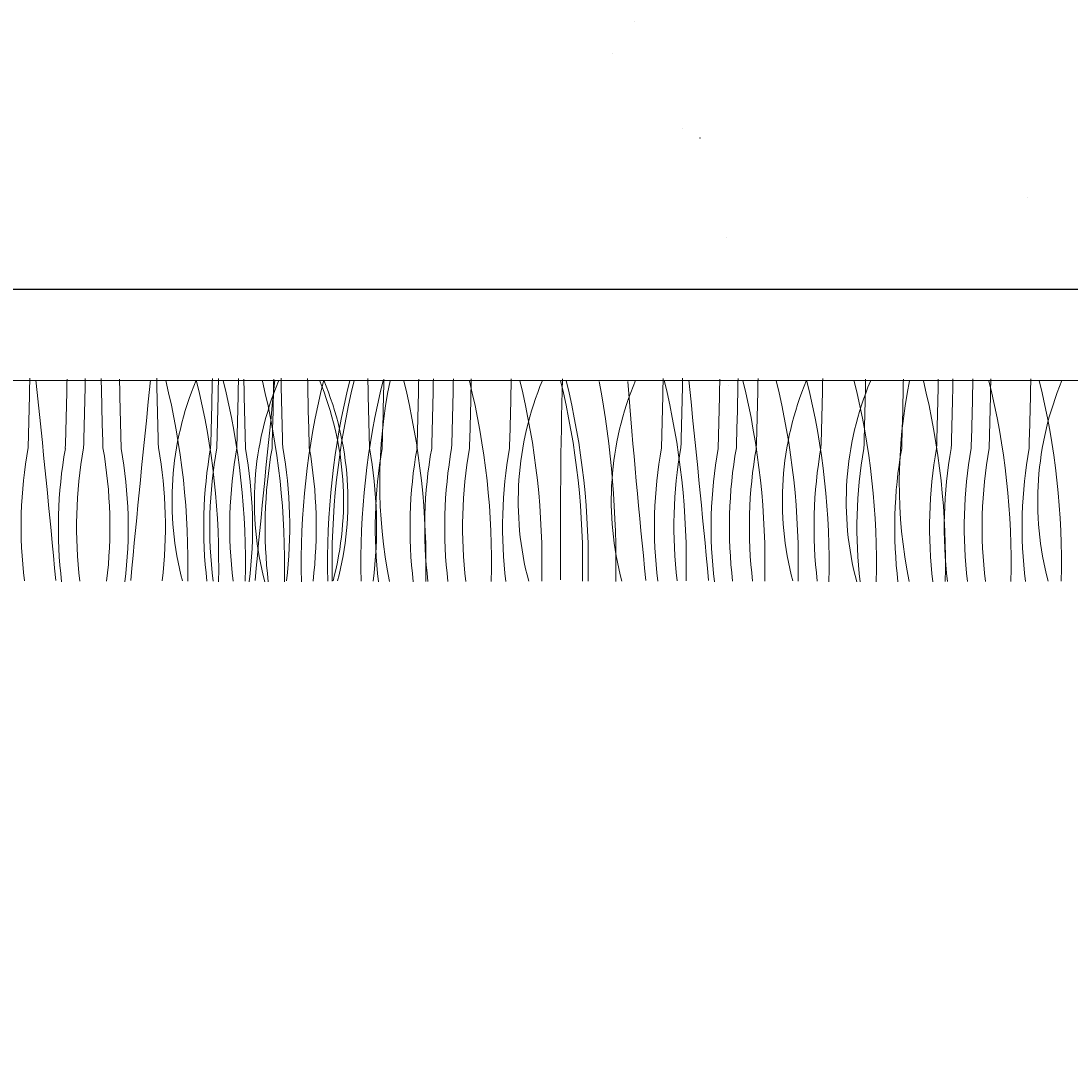
# Model space of a CAD drawing. Units: inches. Extents: x 182 to 1022, y -617 to 111.
# Tile 7 of 33: x 334 to 363, y -310 to -281. Entities that reach past the tile are written whole.
import ezdxf

# ---------------------------------------------------------------- set-up
doc = ezdxf.new("R2010")
doc.units = ezdxf.units.IN
doc.header["$MEASUREMENT"] = 0
doc.layers.add('A-ANNO-DIMS', color=2, linetype='Continuous', lineweight=18)
doc.layers.add('furniture', color=50, linetype='Continuous', lineweight=15, transparency=0.8)
doc.styles.get("Standard").update_dxf_attribs({"font": 'arial.ttf'})
doc.dimstyles.get("Standard").update_dxf_attribs({"dimtxt": 0.18, "dimasz": 0.18, "dimexe": 0.18, "dimexo": 0.0625, "dimgap": 0.09, "dimtad": 0, "dimtih": 1, "dimtoh": 1, "dimdec": 1, "dimzin": 0, "dimdsep": 46, "dimlunit": 4, "dimtxsty": 'Standard', "dimcen": 0.09, "dimadec": 0, "dimazin": 0, "dimtfac": 1, "dimtdec": 1, "dimtofl": 0, "dimtmove": 0, "dimatfit": 3, "dimfxl": 1, "dimtolj": 1, "dimtzin": 0, "dimarcsym": 0})

# ---------------------------------------------------------------- blocks, each defined once
blk = doc.blocks.new('LOUNGE-SEATING-GROUP')
for p, q in [((93.215, 15.865), (93.215, 15.865)), ((93.215, 15.865), (93.215, 15.865)), ((92.603, 14.941), (92.603, 14.941)), ((92.603, 14.941), (92.603, 14.941)), ((94.584, 12.827), (94.584, 12.827)), ((104.328, 10.867), (104.328, 10.867)), ((95.804, 9.742), (95.804, 9.742)), ((134.145, 5.694), (21.664, 5.694)), ((39.442, 5.694), (134.145, 5.694)), ((95.867, 5.548), (95.867, 5.548)), ((81.923, 3.919), (81.923, 3.919)), ((85.76, 3.919), (85.76, 3.919)), ((85.885, 3.919), (85.885, 3.919))]:
    blk.add_line(p, q)
for centre, radius, start, end in [((-66.582, 8.311), 142.714, 358.18909, 358.97752), ((-399.563, -44.164), 478.452, 5.30083, 5.98346), ((-65.529, 8.28), 142.714, 358.18909, 358.97752), ((-65.013, 8.298), 142.714, 358.18909, 358.97752), ((220.821, 8.298), 142.714, 181.02248, 181.81091), ((221.338, 8.28), 142.714, 181.02248, 181.81091), ((555.371, -44.164), 478.452, 174.01654, 174.69917), ((222.39, 8.311), 142.714, 181.02248, 181.81091), ((59.027, 0.538), 21.554, 358.6331, 13.8573), ((88.968, 2.293), 8.837, 157.3098, 194.8613), ((59.898, 0.518), 21.554, 358.6331, 13.8573), ((-61.419, 8.298), 142.714, 358.18909, 358.97752), ((-61.245, 8.298), 142.714, 358.18909, 358.97752), ((60.655, 0.535), 21.554, 358.6331, 13.8573), ((-60.68, 8.299), 142.714, 358.18909, 358.97752), ((224.855, 8.28), 142.714, 181.02248, 181.81091), ((91.298, 2.27), 8.837, 157.3098, 194.8613), ((558.888, -44.164), 478.452, 174.01654, 174.69917), ((61.761, 0.516), 21.554, 358.6331, 13.8573), ((-59.682, 8.279), 142.714, 358.18909, 358.97752), ((225.907, 8.311), 142.714, 181.02248, 181.81091), ((105.341, 0.518), 21.554, 166.1427, 181.3669), ((226.658, 8.298), 142.714, 181.02248, 181.81091), ((76.146, 2.293), 8.837, 345.1387, 22.6902), ((76.271, 2.293), 8.837, 345.1387, 22.6902), ((106.087, 0.538), 21.554, 166.1427, 181.3669), ((106.212, 0.538), 21.554, 166.1427, 181.3669), ((107.028, 0.535), 21.554, 166.1427, 181.3669), ((228.363, 8.299), 142.714, 181.02248, 181.81091), ((100.34, 2.803), 14.333, 168.4112, 191.2455), ((-56.567, 8.282), 142.714, 358.18909, 358.97752), ((65.762, 0.521), 21.554, 358.6331, 13.8573), ((-55.581, 8.285), 142.714, 358.18909, 358.97752), ((-55.166, 8.286), 142.714, 358.18909, 358.97752), ((-54.601, 8.287), 142.714, 358.18909, 358.97752), ((67.616, 0.526), 21.554, 358.6331, 13.8573), ((-54.095, 8.289), 142.714, 358.18909, 358.97752), ((-52.964, 8.292), 142.714, 358.18909, 358.97752), ((98.762, 2.285), 8.837, 157.3098, 194.8613), ((69.042, 0.53), 21.554, 358.6331, 13.8573), ((70.193, 0.531), 21.554, 358.6331, 13.8573), ((275.642, 1.329), 184.521, 178.62796, 180.39341), ((70.354, 0.532), 21.554, 358.6331, 13.8573), ((64.068, 0.5), 28.62, 359.0195, 10.4039), ((101.395, 2.289), 8.837, 157.3098, 194.8613), ((343.842, 25.472), 251.596, 184.51462, 185.80171), ((-48.667, 8.303), 142.714, 358.18909, 358.97752), ((73.125, 0.541), 21.554, 358.6331, 13.8573), ((-48.116, 8.311), 142.714, 358.18909, 358.97752), ((-381.097, -44.164), 478.452, 5.30083, 5.98346), ((-47.064, 8.28), 142.714, 358.18909, 358.97752), ((-46.547, 8.298), 142.714, 358.18909, 358.97752), ((75.352, 0.535), 21.554, 358.6331, 13.8573), ((-45.982, 8.299), 142.714, 358.18909, 358.97752), ((76.294, 0.538), 21.554, 358.6331, 13.8573), ((106.234, 2.293), 8.837, 157.3098, 194.8613), ((77.164, 0.518), 21.554, 358.6331, 13.8573), ((-44.153, 8.298), 142.714, 358.18909, 358.97752), ((108.041, 2.27), 8.837, 157.3098, 194.8613), ((78.503, 0.516), 21.554, 358.6331, 13.8573), ((-42.939, 8.279), 142.714, 358.18909, 358.97752), ((115.038, 2.803), 14.333, 168.4112, 191.2455), ((-41.87, 8.282), 142.714, 358.18909, 358.97752), ((80.459, 0.521), 21.554, 358.6331, 13.8573), ((-40.884, 8.285), 142.714, 358.18909, 358.97752), ((-40.469, 8.286), 142.714, 358.18909, 358.97752), ((-39.904, 8.287), 142.714, 358.18909, 358.97752), ((82.313, 0.526), 21.554, 358.6331, 13.8573), ((-39.398, 8.289), 142.714, 358.18909, 358.97752), ((-38.267, 8.292), 142.714, 358.18909, 358.97752), ((113.459, 2.285), 8.837, 157.3098, 194.8613), ((83.739, 0.53), 21.554, 358.6331, 13.8573), ((88.658, 1.565), 12.794, 169.9349, 186.8829), ((89.711, 1.534), 12.794, 169.9349, 186.8829), ((90.227, 1.552), 12.794, 169.9349, 186.8829), ((65.581, 1.552), 12.794, 353.1171, 10.0651), ((66.098, 1.534), 12.794, 353.1171, 10.0651), ((67.15, 1.565), 12.794, 353.1171, 10.0651), ((93.821, 1.552), 12.794, 169.9349, 186.8829), ((93.995, 1.552), 12.794, 169.9349, 186.8829), ((94.56, 1.553), 12.794, 169.9349, 186.8829), ((69.615, 1.534), 12.794, 353.1171, 10.0651), ((95.558, 1.534), 12.794, 169.9349, 186.8829), ((70.667, 1.565), 12.794, 353.1171, 10.0651), ((71.418, 1.552), 12.794, 353.1171, 10.0651), ((73.123, 1.553), 12.794, 353.1171, 10.0651), ((98.673, 1.536), 12.794, 169.9349, 186.8829), ((99.659, 1.539), 12.794, 169.9349, 186.8829), ((100.074, 1.54), 12.794, 169.9349, 186.8829), ((100.639, 1.542), 12.794, 169.9349, 186.8829), ((101.145, 1.543), 12.794, 169.9349, 186.8829), ((102.276, 1.546), 12.794, 169.9349, 186.8829), ((106.573, 1.557), 12.794, 169.9349, 186.8829), ((107.124, 1.565), 12.794, 169.9349, 186.8829), ((108.176, 1.534), 12.794, 169.9349, 186.8829), ((108.693, 1.552), 12.794, 169.9349, 186.8829), ((109.258, 1.553), 12.794, 169.9349, 186.8829), ((111.087, 1.552), 12.794, 169.9349, 186.8829), ((112.301, 1.534), 12.794, 169.9349, 186.8829), ((113.37, 1.536), 12.794, 169.9349, 186.8829), ((114.356, 1.539), 12.794, 169.9349, 186.8829), ((114.771, 1.54), 12.794, 169.9349, 186.8829), ((115.336, 1.542), 12.794, 169.9349, 186.8829), ((115.842, 1.543), 12.794, 169.9349, 186.8829), ((116.973, 1.546), 12.794, 169.9349, 186.8829)]:
    blk.add_arc(centre, radius, start, end)
blk.add_point((95.069, 12.557))
blk = doc.blocks.new('*D26')
at = {"layer": 'A-ANNO-DIMS', "color": 0, "lineweight": -2, "transparency": 16777216}
for p, q in [((257.848, -296.884), (257.848, -319.733)), ((409.388, -296.884), (409.388, -319.733)), ((258.028, -319.553), (331.642, -319.553)), ((409.208, -319.553), (335.594, -319.553))]:
    blk.add_line(p, q, dxfattribs=at)
at = {"layer": 'A-ANNO-DIMS', "color": 0, "transparency": 16777216}
for points in [[(258.028, -319.523), (258.028, -319.583), (257.848, -319.553)], [(409.208, -319.523), (409.208, -319.583), (409.388, -319.553)]]:
    blk.add_solid(points, dxfattribs=at)
at = {"layer": 'Defpoints', "color": 0, "transparency": 16777216}
for p in [(257.848, -296.822), (409.388, -296.822), (409.388, -319.553)]:
    blk.add_point(p, dxfattribs=at)
at = {"layer": 'A-ANNO-DIMS', "color": 0, "transparency": 16777216, "insert": (333.618, -319.553), "char_height": 0.18, "attachment_point": 5}
blk.add_mtext('\\A1;LOUNGE GROUP 12\'-7 1/2" TYP.', dxfattribs=at)
blk = doc.blocks.new('*D39')
at = {"layer": 'A-ANNO-DIMS', "color": 0, "lineweight": -2, "transparency": 16777216}
for p, q in [((238.398, -288.54), (1015.285, -288.54)), ((1015.105, -288.72), (1015.105, -346.775)), ((1015.105, -405.193), (1015.105, -347.138)), ((238.427, -405.373), (1015.285, -405.373))]:
    blk.add_line(p, q, dxfattribs=at)
at = {"layer": 'A-ANNO-DIMS', "color": 0, "transparency": 16777216}
for points in [[(1015.075, -288.72), (1015.135, -288.72), (1015.105, -288.54)], [(1015.075, -405.193), (1015.135, -405.193), (1015.105, -405.373)]]:
    blk.add_solid(points, dxfattribs=at)
at = {"layer": 'Defpoints', "color": 0, "transparency": 16777216}
for p in [(238.335, -288.54), (1015.105, -288.54), (238.364, -405.373)]:
    blk.add_point(p, dxfattribs=at)
at = {"layer": 'A-ANNO-DIMS', "color": 0, "transparency": 16777216, "insert": (1015.105, -346.956), "char_height": 0.18, "attachment_point": 5}
blk.add_mtext('\\A1;9\'-9"', dxfattribs=at)

msp = doc.modelspace()

# ---------------------------------------------------------------- block references
at = {"layer": 'furniture'}
msp.add_blockref('LOUNGE-SEATING-GROUP', (257.848, -296.822), dxfattribs=at)

# ---------------------------------------------------------------- dimensions: what is measured, and where the dimension line sits
at = {"layer": 'A-ANNO-DIMS'}
dim = msp.add_linear_dim(base=(1015.105, -288.54), p1=(238.364, -405.373), p2=(238.335, -288.54), angle=90, dimstyle='Standard', override={"dimdec": 1, "dimlfac": 1, "dimrnd": 0, "dimzin": 1, "dimdsep": 46, "dimlunit": 4, "dimfrac": 2}, dxfattribs=at)
dim.commit()
dim.dimension.update_dxf_attribs({"geometry": '*D39', "text_midpoint": (1015.105, -346.956)})
dim = msp.add_linear_dim(base=(409.388, -319.553), p1=(257.848, -296.822), p2=(409.388, -296.822), text='LOUNGE GROUP <> TYP.', dimstyle='Standard', override={"dimdec": 1, "dimlfac": 1, "dimrnd": 0, "dimzin": 1, "dimdsep": 46, "dimlunit": 4, "dimfrac": 2}, dxfattribs=at)
dim.commit()
dim.dimension.update_dxf_attribs({"geometry": '*D26', "text_midpoint": (333.618, -319.553)})

doc.saveas('drawing.dxf')
